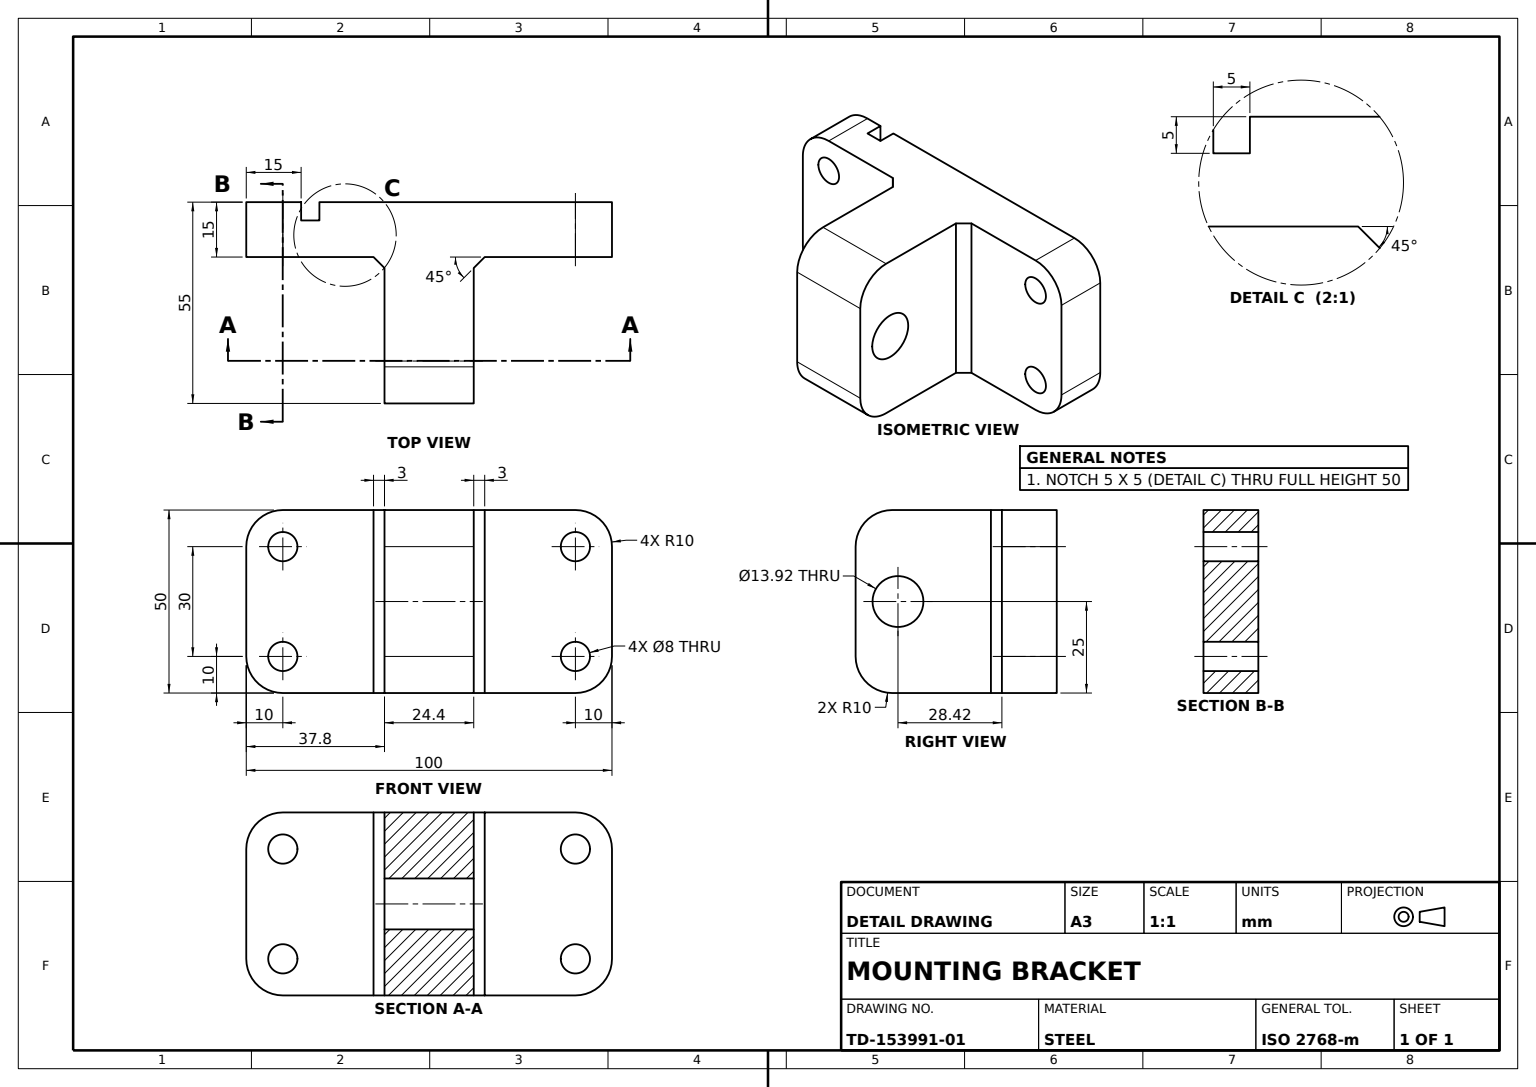
SolidWorks part; units mm, degrees
material "Plain Carbon Steel"
ref_plane "Front Plane" through (0, 0, 0) normal (0, 0, 1) x (1, 0, 0)
ref_plane "Top Plane" through (0, 0, 0) normal (0, 1, 0) x (1, 0, 0)
ref_plane "Right Plane" through (0, 0, 0) normal (1, 0, 0) x (0, 0, -1)
sketch "Base Plate Sketch" plane through (0, 0, 0) normal (0, 0, 1) x (1, 0, 0)
  line L0 (10, 0) -> (90, 0)
  line L1 (100, 10) -> (100, 40)
  line L2 (90, 50) -> (10, 50)
  line L3 (0, 40) -> (0, 10)
  arc A0 (100, 40) -> (90, 50) centre (90, 40) ccw
  arc A1 (90, 0) -> (100, 10) centre (90, 10) ccw
  arc A2 (10, 0) -> (0, 10) centre (10, 10) cw
  arc A3 (10, 50) -> (0, 40) centre (10, 40) ccw
  point P11 (0, 0)
  dimension "D1" = 10
  dimension "D2" = 10
  dimension "D3" = 10
  dimension "D4" = 10
  dimension "D5" = 100
  dimension "D6" = 50
extrude "Base Plate" add sketch "Base Plate Sketch" along normal blind 15
sketch "Knuckle Block Sketch" plane through (100, 0, 0) normal (1, 0, 0) x (0, 0, -1)
  line L0 (-15, 50) -> (-45, 50)
  line L1 (-55, 40) -> (-55, 10)
  line L2 (-45, 0) -> (-15, 0)
  line L3 (-15, 50) -> (-15, 0)
  arc A0 (-55, 40) -> (-45, 50) centre (-45, 40) cw
  arc A1 (-55, 10) -> (-45, 0) centre (-45, 10) ccw
  dimension "D1" = 10
  dimension "D2" = 10
  dimension "D3" = 40
extrude "Knuckle Block" add sketch "Knuckle Block Sketch" against normal blind 100
sketch "Knuckle Relief Cut A Sketch" plane through (100, 0, 0) normal (1, 0, 0) x (0, 0, -1)
  line L0 (-15, 40) -> (-15, 50)
  line L1 (-15, 50) -> (-45, 50)
  line L3 (-45, 0) -> (-15, 0)
  line L4 (-15, 0) -> (-15, 40)
  line L5 (-55, 40) -> (-55, 10)
  arc A0 (-45, 50) -> (-55, 40) centre (-45, 40) ccw
  arc A1 (-55, 10) -> (-45, 0) centre (-45, 10) ccw
extrude "Knuckle Relief Cut A" cut sketch "Knuckle Relief Cut A Sketch" against normal blind 37.8
sketch "Knuckle Relief Cut B Sketch" plane through (0, 0, 0) normal (-1, 0, 0) x (0, 0, 1)
  line L0 (15, 50) -> (45, 50)
  line L1 (15, 50) -> (15, 0)
  line L2 (15, 0) -> (45, 0)
  line L3 (55, 40) -> (55, 10)
  arc A0 (55, 40) -> (45, 50) centre (45, 40) ccw
  arc A1 (45, 0) -> (55, 10) centre (45, 10) ccw
extrude "Knuckle Relief Cut B" cut sketch "Knuckle Relief Cut B Sketch" against normal blind 37.8
sketch "Plate Mounting Holes Sketch" plane through (0, 0, 0) normal (0, -1, 0) x (1, 0, 0)
  line L0 (10, 15) -> (10, 0) construction
  line L1 (10, 0) -> (90, 0) construction
  line L2 (15, 0) -> (15, 5)
  line L3 (15, 5) -> (20, 5)
  line L4 (20, 5) -> (20, 0)
  line L5 (20, 0) -> (15, 0)
  dimension "D1" = 5
  dimension "D2" = 10
extrude "Plate Mounting Holes" cut sketch "Plate Mounting Holes Sketch" against normal blind 50
sketch "Hinge Pin Hole Sketch" plane through (62.2, 0, 0) normal (1, 0, 0) x (0, 0, -1)
  line L0 (-15, 50) -> (-45, 50) construction
  line L1 (-15, 0) -> (-15, 50) construction
  circle A0 centre (-43.416, 25) radius 6.958
  dimension "D1" = 13.9159
  dimension "D2" = 28.416
  dimension "D3" = 25
extrude "Hinge Pin Hole" cut sketch "Hinge Pin Hole Sketch" against normal blind 50
sketch "Upper Mounting Holes Sketch" plane through (0, 0, 15) normal (0, 0, 1) x (1, 0, 0)
  circle A0 centre (90, 40) radius 4
  circle A1 centre (90, 10) radius 4
  circle A2 centre (10, 40) radius 4
  circle A3 centre (10, 10) radius 4
  dimension "D1" = 8
extrude "Upper Mounting Holes" cut sketch "Upper Mounting Holes Sketch" against normal blind 50
chamfer "Knuckle Chamfer A 3x45" distance 3 angle 45 1 edges at (62.2, 25, 15)
chamfer "Knuckle Chamfer B 3x45" distance 3 angle 45 1 edges at (37.8, 25, 15)
